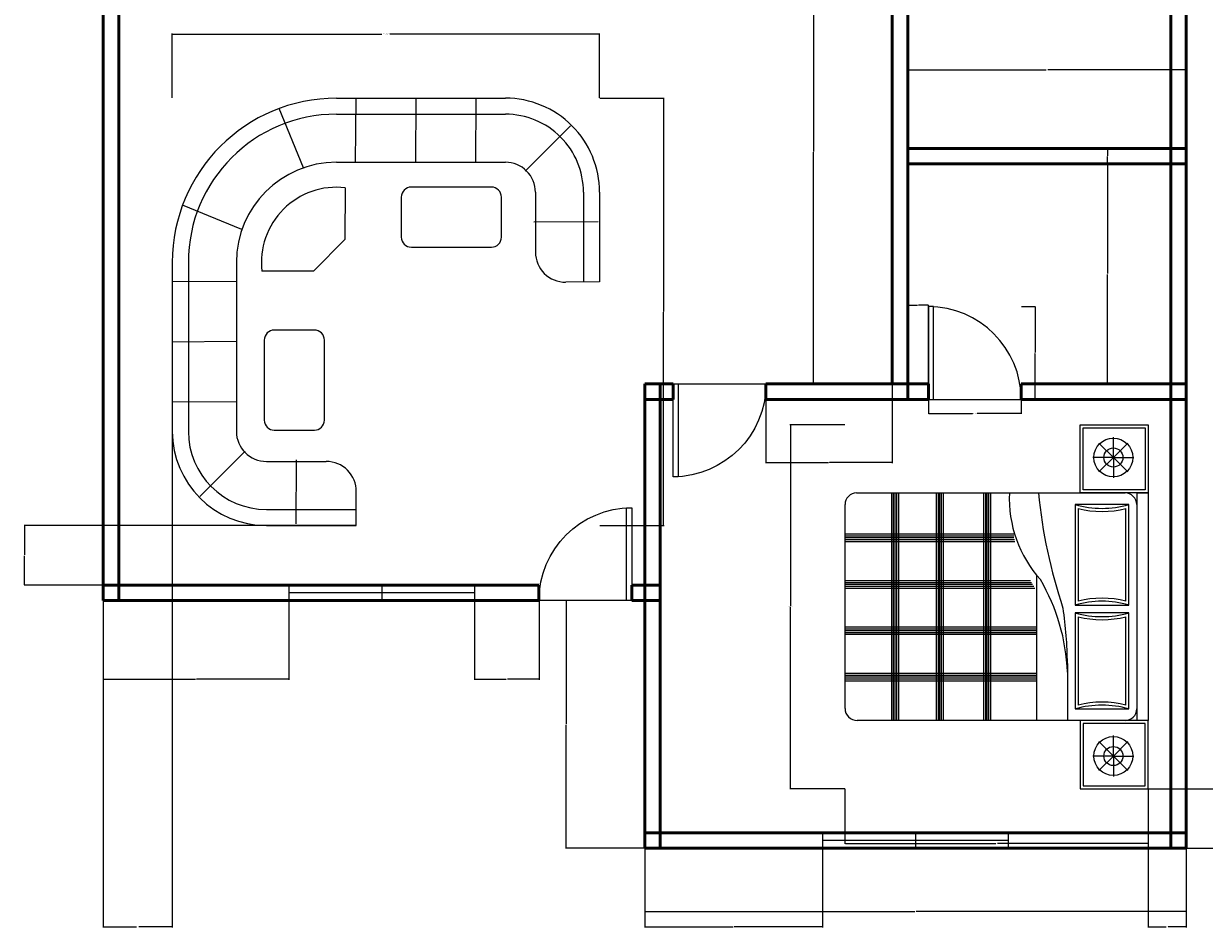
# Model space of a CAD drawing. Units: inches. Extents: x 224 to 929, y 339 to 940.
# Tile 1 of 3: x 224 to 682, y 339 to 689. Entities that reach past the tile are written whole.
import ezdxf

# ---------------------------------------------------------------- set-up
doc = ezdxf.new("R2010")
doc.units = ezdxf.units.IN
for name, color, linetype, lineweight in [('A-ANNO-DIMS', 2, 'Continuous', 18), ('A-DOOR', 3, 'Continuous', 25), ('A-FURN', 8, 'Continuous', 18), ('A-GLAZ', 4, 'Continuous', 18), ('A-WALL', 7, 'Continuous', 50)]:
    doc.layers.add(name, color=color, linetype=linetype, lineweight=lineweight)
doc.styles.get("Standard").update_dxf_attribs({"font": 'arial.ttf'})
doc.dimstyles.get("Standard").update_dxf_attribs({"dimtxt": 0.18, "dimasz": 0.18, "dimexe": 0.18, "dimexo": 0.0625, "dimgap": 0.09, "dimtad": 0, "dimtih": 1, "dimtoh": 1, "dimdec": 4, "dimzin": 0, "dimdsep": 46, "dimtxsty": 'Standard', "dimcen": 0.09, "dimadec": 0, "dimazin": 0, "dimtfac": 1, "dimtdec": 4, "dimtofl": 0, "dimtmove": 0, "dimatfit": 3, "dimfxl": 1, "dimtolj": 1, "dimtzin": 0, "dimarcsym": 0})

# ---------------------------------------------------------------- blocks, each defined once
blk = doc.blocks.new('A$C2EB62172')
at = {"linetype": 'ByBlock'}
for p, q in [((0, 2.0003), (0.45, 2.0003)), ((0, 1.5503), (0, 2.0003)), ((0.45, 1.9241), (0.45, 2.0003)), ((0.45, 2.0003), (0.45, 1.5503)), ((0.45, 2.0003), (1.9506, 2.0003)), ((1.9506, 2.0003), (1.9506, 1.5503)), ((2.4006, 2.0003), (1.9506, 2.0003)), ((2.4006, 1.5503), (2.4006, 2.0003)), ((0.45, 1.9241), (1.9506, 1.9241)), ((0.45, 0.0763), (0.45, 1.8479)), ((1.9506, 1.8479), (1.9506, 0.0801)), ((0.45, 1.5503), (0, 1.5503)), ((1.9506, 1.5503), (2.4006, 1.5503)), ((1.8706, 0.0001), (0.5262, 0.0001))]:
    blk.add_line(p, q, dxfattribs=at)
for p, q in [((0.02, 1.9803), (0.43, 1.9803)), ((0.02, 1.5703), (0.02, 1.9803)), ((0.43, 1.9803), (0.43, 1.5703)), ((1.9706, 1.9803), (1.9706, 1.5703)), ((2.3806, 1.9803), (1.9706, 1.9803)), ((2.3806, 1.5703), (2.3806, 1.9803)), ((0.2161, 1.7703), (0.2161, 1.9047)), ((0.5262, 1.8733), (0.5262, 1.5177)), ((1.1893, 1.8733), (0.5262, 1.8733)), ((1.1893, 1.5177), (1.1893, 1.8733)), ((1.2401, 1.8733), (1.2401, 1.5177)), ((1.8744, 1.8733), (1.2401, 1.8733)), ((1.8744, 1.5177), (1.8744, 1.8733)), ((2.1846, 1.7703), (2.1846, 1.9047)), ((0.2161, 1.7703), (0.1211, 1.8653)), ((0.2161, 1.7703), (0.3111, 1.8653)), ((1.1632, 1.8533), (0.5523, 1.8533)), ((1.8483, 1.8533), (1.2662, 1.8533)), ((2.1846, 1.7703), (2.0896, 1.8653)), ((2.1846, 1.7703), (2.2796, 1.8653)), ((0.2161, 1.7703), (0.0817, 1.7703)), ((0.2161, 1.7703), (0.1211, 1.6753)), ((0.2161, 1.7703), (0.3505, 1.7703)), ((0.2161, 1.7703), (0.3111, 1.6753)), ((0.2161, 1.7703), (0.2161, 1.6359)), ((2.1846, 1.7703), (2.0502, 1.7703)), ((2.1846, 1.7703), (2.0896, 1.6753)), ((2.1846, 1.7703), (2.1846, 1.6359)), ((2.1846, 1.7703), (2.319, 1.7703)), ((2.1846, 1.7703), (2.2796, 1.6753)), ((0.43, 1.5703), (0.02, 1.5703)), ((1.9706, 1.5703), (2.3806, 1.5703)), ((0.5262, 1.5177), (1.1893, 1.5177)), ((0.5523, 1.5377), (1.1632, 1.5377)), ((1.2401, 1.5177), (1.8744, 1.5177)), ((1.2662, 1.5377), (1.8483, 1.5377)), ((1.5747, 1.4669), (1.9506, 1.4669)), ((0.996, 1.2637), (1.9506, 1.2637)), ((1.079, 1.2529), (1.079, 0.0001)), ((1.3351, 1.2637), (1.3351, 0.0001)), ((1.3471, 1.2637), (1.3471, 0.0001)), ((1.3591, 1.2637), (1.3591, 0.0001)), ((1.3722, 1.2637), (1.3722, 0.0001)), ((1.3842, 1.2637), (1.3842, 0.0001)), ((1.6409, 1.2637), (1.6409, 0.0001)), ((1.6529, 1.2637), (1.6529, 0.0001)), ((1.6649, 1.2637), (1.6649, 0.0001)), ((1.678, 1.2637), (1.678, 0.0001)), ((1.69, 1.2637), (1.69, 0.0001)), ((1.0299, 1.2232), (1.0299, 0.0001)), ((1.0419, 1.2301), (1.0419, 0.0001)), ((1.0539, 1.2373), (1.0539, 0.0001)), ((1.067, 1.2453), (1.067, 0.0001)), ((0.722, 1.1147), (0.722, 0.0001)), ((0.734, 1.1147), (0.734, 0.0001)), ((0.746, 1.1147), (0.746, 0.0001)), ((0.7591, 1.1172), (0.7591, 0.0001)), ((0.7711, 1.1203), (0.7711, 0.0001)), ((0.45, 0.9593), (1.9506, 0.9593)), ((0.45, 0.9473), (1.9506, 0.9473)), ((0.45, 0.9353), (1.9506, 0.9353)), ((0.45, 0.9259), (1.9506, 0.9259)), ((0.45, 0.9139), (1.9506, 0.9139)), ((0.45, 0.6471), (1.9506, 0.6471)), ((0.45, 0.6351), (1.9506, 0.6351)), ((0.45, 0.6231), (1.9506, 0.6231)), ((0.45, 0.6137), (1.9506, 0.6137)), ((0.45, 0.6017), (1.9506, 0.6017)), ((0.45, 0.3522), (1.9506, 0.3522)), ((0.45, 0.3402), (1.9506, 0.3402)), ((0.45, 0.3282), (1.9506, 0.3282)), ((0.45, 0.3188), (1.9506, 0.3188)), ((0.45, 0.3068), (1.9506, 0.3068))]:
    blk.add_line(p, q)
for centre, radius in [((0.2161, 1.7703), 0.1285), ((2.1846, 1.7703), 0.1285), ((0.2161, 1.7703), 0.0628), ((2.1846, 1.7703), 0.0628)]:
    blk.add_circle(centre, radius)
for centre, radius, start, end in [((0.5262, 1.8479), 0.0762, 90, 180), ((1.8744, 1.8479), 0.0762, 0, 90), ((1.8706, 0.0801), 0.08, 270, 0), ((0.5262, 0.0763), 0.0762, 180, 270)]:
    blk.add_arc(centre, radius, start, end, dxfattribs=at)
for centre, radius, start, end in [((-0.0834, 1.6955), 0.635, 343.73979, 16.26021), ((1.7989, 1.6955), 0.635, 163.73979, 196.26021), ((0.6305, 1.6955), 0.635, 343.73979, 16.26021), ((2.484, 1.6955), 0.635, 163.73979, 196.26021), ((-0.0834, 1.6955), 0.655, 346.05939, 13.94061), ((1.7989, 1.6955), 0.655, 166.05939, 193.94061), ((0.6305, 1.6955), 0.655, 346.05939, 13.94061), ((2.484, 1.6955), 0.655, 166.05939, 193.94061), ((0.1114, 4.7131), 3.454, 275.6242, 288.5258), ((1.6775, 0.1733), 1.2944, 92.03201, 120.45698), ((1.5739, -0.8648), 2.3317, 89.98016, 99.00664), ((0.4851, 1.8866), 0.8029, 267.49694, 311.91323)]:
    blk.add_arc(centre, radius, start, end)
blk = doc.blocks.new('A$C0BCD5431')
for p, q in [((2628, 4268), (940, 4268)), ((1236, 4268), (1240, 3628)), ((1836, 4268), (1840, 3628)), ((2436, 4268), (2440, 3628)), ((2957, 3573), (3201, 4165)), ((2628, 4108), (940, 4108)), ((742, 3540), (290, 3993)), ((2628, 3628), (940, 3628)), ((0, 3328), (0, 2432)), ((160, 3328), (160, 2431)), ((640, 3328), (640, 2730)), ((1852, 3349), (1052, 3349)), ((2542, 3373), (2545, 2855)), ((952, 3249), (952, 2849)), ((1952, 2849), (1952, 3249)), ((3573, 2957), (4165, 3201)), ((15, 3032), (655, 3028)), ((2545, 2855), (2855, 2545)), ((1052, 2749), (1852, 2749)), ((3628, 2628), (3628, 940)), ((4108, 2628), (4108, 940)), ((4268, 2628), (4268, 940)), ((3373, 2542), (2855, 2545)), ((0, 2432), (338, 2430)), ((4268, 2436), (3628, 2440)), ((3280, 1980), (2880, 1980)), ((2780, 1880), (2780, 1080)), ((3380, 1080), (3380, 1880)), ((4268, 1836), (3628, 1840)), ((4268, 1236), (3628, 1240)), ((2880, 980), (3280, 980)), ((3540, 742), (3993, 290)), ((3328, 640), (2730, 640)), ((3032, 15), (3028, 655)), ((2432, 0), (2430, 338)), ((3328, 160), (2431, 160)), ((3328, 0), (2432, 0))]:
    blk.add_line(p, q)
for centre, radius, start, end in [((940, 3328), 940, 90, 180), ((2628, 2628), 1640, 0, 90), ((940, 3328), 780, 90, 180), ((2628, 2628), 1480, 0, 90), ((940, 3328), 300, 90, 180), ((2628, 2628), 1000, 0, 90), ((1052, 3249), 100, 90, 180), ((1852, 3249), 100, 0, 90), ((2628, 2628), 750, 353.3601, 96.6399), ((1052, 2849), 100, 180, 270), ((1852, 2849), 100, 270, 0), ((340, 2730), 300, 269.6481, 0), ((2880, 1880), 100, 90, 180), ((3280, 1880), 100, 0, 90), ((2880, 1080), 100, 180, 270), ((3280, 1080), 100, 270, 0), ((3328, 940), 300, 270, 0), ((3328, 940), 780, 270, 0), ((3328, 940), 940, 270, 0), ((2730, 340), 300, 90, 180.3519)]:
    blk.add_arc(centre, radius, start, end)
blk = doc.blocks.new('DOOR-SINGLE-36IN')
blk.add_line((0, 0), (36, 0))
blk.add_lwpolyline([(2, 0), (2, 36), (0, 36), (0, 0)], close=True)
blk.add_arc((0, 0), 36, 0, 90)
blk = doc.blocks.new('WIN-72IN')
for p, q in [((0, 0), (0, 6)), ((36, 0), (36, 6)), ((72, 0), (72, 6)), ((0, 3), (72, 3))]:
    blk.add_line(p, q)
blk = doc.blocks.new('*D5')
at = {"layer": 'A-ANNO-DIMS', "color": 0, "lineweight": -2, "transparency": 16777216}
for p, q in [((574.67, 543.56), (574.67, 538.05)), ((610.67, 543.56), (610.67, 538.05)), ((574.85, 538.23), (591.73, 538.23)), ((610.49, 538.23), (593.6, 538.23))]:
    blk.add_line(p, q, dxfattribs=at)
at = {"layer": 'A-ANNO-DIMS', "color": 0, "transparency": 16777216}
for points in [[(574.85, 538.26), (574.85, 538.2), (574.67, 538.23)], [(610.49, 538.26), (610.49, 538.2), (610.67, 538.23)]]:
    blk.add_solid(points, dxfattribs=at)
at = {"layer": 'Defpoints', "color": 0, "transparency": 16777216}
for p in [(574.67, 543.63), (610.67, 543.63), (610.67, 538.23)]:
    blk.add_point(p, dxfattribs=at)
at = {"layer": 'A-ANNO-DIMS', "color": 0, "transparency": 16777216, "insert": (592.67, 538.23), "char_height": 0.18, "attachment_point": 5}
blk.add_mtext('\\A1;DOOR 36 TYP.', dxfattribs=at)
blk = doc.blocks.new('*D6')
at = {"layer": 'A-ANNO-DIMS', "color": 0, "lineweight": -2, "transparency": 16777216}
for p, q in [((610.73, 579.63), (616.25, 579.63)), ((616.07, 579.45), (616.07, 561.81)), ((616.07, 543.81), (616.07, 561.44)), ((610.73, 543.63), (616.25, 543.63))]:
    blk.add_line(p, q, dxfattribs=at)
at = {"layer": 'A-ANNO-DIMS', "color": 0, "transparency": 16777216}
for points in [[(616.04, 579.45), (616.1, 579.45), (616.07, 579.63)], [(616.04, 543.81), (616.1, 543.81), (616.07, 543.63)]]:
    blk.add_solid(points, dxfattribs=at)
at = {"layer": 'Defpoints', "color": 0, "transparency": 16777216}
for p in [(610.67, 579.63), (616.07, 579.63), (610.67, 543.63)]:
    blk.add_point(p, dxfattribs=at)
at = {"layer": 'A-ANNO-DIMS', "color": 0, "transparency": 16777216, "insert": (616.07, 561.63), "char_height": 0.18, "attachment_point": 5}
blk.add_mtext('\\A1;36 TYP.', dxfattribs=at)
blk = doc.blocks.new('*D11')
at = {"layer": 'A-ANNO-DIMS', "color": 0, "lineweight": -2, "transparency": 16777216}
for p, q in [((542.28, 533.81), (520.99, 533.81)), ((521.17, 533.63), (521.17, 463.43)), ((521.17, 392.86), (521.17, 463.06)), ((542.28, 392.68), (520.99, 392.68))]:
    blk.add_line(p, q, dxfattribs=at)
at = {"layer": 'A-ANNO-DIMS', "color": 0, "transparency": 16777216}
for points in [[(521.14, 533.63), (521.2, 533.63), (521.17, 533.81)], [(521.14, 392.86), (521.2, 392.86), (521.17, 392.68)]]:
    blk.add_solid(points, dxfattribs=at)
at = {"layer": 'Defpoints', "color": 0, "transparency": 16777216}
for p in [(542.34, 533.81), (521.17, 392.68), (542.34, 392.68)]:
    blk.add_point(p, dxfattribs=at)
at = {"layer": 'A-ANNO-DIMS', "color": 0, "transparency": 16777216, "insert": (521.17, 463.25), "char_height": 0.18, "attachment_point": 5}
blk.add_mtext('\\A1;BED GROUP 141', dxfattribs=at)
blk = doc.blocks.new('*D12')
at = {"layer": 'A-ANNO-DIMS', "color": 0, "lineweight": -2, "transparency": 16777216}
for p, q in [((542.34, 392.62), (542.34, 371.33)), ((659.94, 392.62), (659.94, 371.33)), ((542.52, 371.51), (600.86, 371.51)), ((659.76, 371.51), (601.42, 371.51))]:
    blk.add_line(p, q, dxfattribs=at)
at = {"layer": 'A-ANNO-DIMS', "color": 0, "transparency": 16777216}
for points in [[(542.52, 371.54), (542.52, 371.48), (542.34, 371.51)], [(659.76, 371.54), (659.76, 371.48), (659.94, 371.51)]]:
    blk.add_solid(points, dxfattribs=at)
at = {"layer": 'Defpoints', "color": 0, "transparency": 16777216}
for p in [(542.34, 392.68), (659.94, 392.68), (659.94, 371.51)]:
    blk.add_point(p, dxfattribs=at)
at = {"layer": 'A-ANNO-DIMS', "color": 0, "transparency": 16777216, "insert": (601.14, 371.51), "char_height": 0.18, "attachment_point": 5}
blk.add_mtext('\\A1;118', dxfattribs=at)
blk = doc.blocks.new('*D13')
at = {"layer": 'A-ANNO-DIMS', "color": 0, "lineweight": -2, "transparency": 16777216}
for p, q in [((281.45, 660.5), (281.45, 685.47)), ((281.63, 685.29), (362.76, 685.29)), ((446.95, 685.29), (365.82, 685.29)), ((447.13, 660.5), (447.13, 685.47))]:
    blk.add_line(p, q, dxfattribs=at)
at = {"layer": 'A-ANNO-DIMS', "color": 0, "transparency": 16777216}
for points in [[(281.63, 685.32), (281.63, 685.26), (281.45, 685.29)], [(446.95, 685.32), (446.95, 685.26), (447.13, 685.29)]]:
    blk.add_solid(points, dxfattribs=at)
at = {"layer": 'Defpoints', "color": 0, "transparency": 16777216}
for p in [(281.45, 685.29), (281.45, 660.43), (447.13, 660.43)]:
    blk.add_point(p, dxfattribs=at)
at = {"layer": 'A-ANNO-DIMS', "color": 0, "transparency": 16777216, "insert": (364.29, 685.29), "char_height": 0.18, "attachment_point": 5}
blk.add_mtext('\\A1;SECTIONAL GROUP 166', dxfattribs=at)
blk = doc.blocks.new('*D14')
at = {"layer": 'A-ANNO-DIMS', "color": 0, "lineweight": -2, "transparency": 16777216}
for p, q in [((447.2, 660.43), (472.16, 660.43)), ((471.98, 660.25), (471.98, 577.77)), ((471.98, 494.93), (471.98, 577.41)), ((447.2, 494.75), (472.16, 494.75))]:
    blk.add_line(p, q, dxfattribs=at)
at = {"layer": 'A-ANNO-DIMS', "color": 0, "transparency": 16777216}
for points in [[(471.95, 660.25), (472.01, 660.25), (471.98, 660.43)], [(471.95, 494.93), (472.01, 494.93), (471.98, 494.75)]]:
    blk.add_solid(points, dxfattribs=at)
at = {"layer": 'Defpoints', "color": 0, "transparency": 16777216}
for p in [(447.13, 660.43), (471.98, 660.43), (447.13, 494.75)]:
    blk.add_point(p, dxfattribs=at)
at = {"layer": 'A-ANNO-DIMS', "color": 0, "transparency": 16777216, "insert": (471.98, 577.59), "char_height": 0.18, "attachment_point": 5}
blk.add_mtext('\\A1;166', dxfattribs=at)
blk = doc.blocks.new('*D16')
at = {"layer": 'A-ANNO-DIMS', "color": 0, "lineweight": -2, "transparency": 16777216}
for p, q in [((668.73, 909.63), (699.35, 909.63)), ((699.17, 909.45), (699.17, 639.81)), ((699.17, 369.81), (699.17, 639.44)), ((668.73, 369.63), (699.35, 369.63))]:
    blk.add_line(p, q, dxfattribs=at)
at = {"layer": 'A-ANNO-DIMS', "color": 0, "transparency": 16777216}
for points in [[(699.14, 909.45), (699.2, 909.45), (699.17, 909.63)], [(699.14, 369.81), (699.2, 369.81), (699.17, 369.63)]]:
    blk.add_solid(points, dxfattribs=at)
at = {"layer": 'Defpoints', "color": 0, "transparency": 16777216}
for p in [(668.67, 909.63), (668.67, 369.63), (699.17, 369.63)]:
    blk.add_point(p, dxfattribs=at)
at = {"layer": 'A-ANNO-DIMS', "color": 0, "transparency": 16777216, "insert": (699.17, 639.63), "char_height": 0.18, "attachment_point": 5}
blk.add_mtext('\\A1;540', dxfattribs=at)
blk = doc.blocks.new('*D20')
at = {"layer": 'A-ANNO-DIMS', "color": 0, "lineweight": -2, "transparency": 16777216}
for p, q in [((464.67, 375.56), (464.67, 344.95)), ((674.67, 375.56), (674.67, 344.95)), ((464.85, 345.13), (569.38, 345.13)), ((674.49, 345.13), (569.96, 345.13))]:
    blk.add_line(p, q, dxfattribs=at)
at = {"layer": 'A-ANNO-DIMS', "color": 0, "transparency": 16777216}
for points in [[(464.85, 345.16), (464.85, 345.1), (464.67, 345.13)], [(674.49, 345.16), (674.49, 345.1), (674.67, 345.13)]]:
    blk.add_solid(points, dxfattribs=at)
at = {"layer": 'Defpoints', "color": 0, "transparency": 16777216}
for p in [(464.67, 375.63), (674.67, 375.63), (464.67, 345.13)]:
    blk.add_point(p, dxfattribs=at)
at = {"layer": 'A-ANNO-DIMS', "color": 0, "transparency": 16777216, "insert": (569.67, 345.13), "char_height": 0.18, "attachment_point": 5}
blk.add_mtext('\\A1;210', dxfattribs=at)
blk = doc.blocks.new('*D21')
at = {"layer": 'A-ANNO-DIMS', "color": 0, "lineweight": -2, "transparency": 16777216}
for p, q in [((464.6, 465.63), (433.99, 465.63)), ((434.17, 465.45), (434.17, 417.81)), ((434.17, 369.81), (434.17, 417.44)), ((464.6, 369.63), (433.99, 369.63))]:
    blk.add_line(p, q, dxfattribs=at)
at = {"layer": 'A-ANNO-DIMS', "color": 0, "transparency": 16777216}
for points in [[(434.14, 465.45), (434.2, 465.45), (434.17, 465.63)], [(434.14, 369.81), (434.2, 369.81), (434.17, 369.63)]]:
    blk.add_solid(points, dxfattribs=at)
at = {"layer": 'Defpoints', "color": 0, "transparency": 16777216}
for p in [(434.17, 465.63), (464.67, 465.63), (464.67, 369.63)]:
    blk.add_point(p, dxfattribs=at)
at = {"layer": 'A-ANNO-DIMS', "color": 0, "transparency": 16777216, "insert": (434.17, 417.63), "char_height": 0.18, "attachment_point": 5}
blk.add_mtext('\\A1;96', dxfattribs=at)
blk = doc.blocks.new('*D22')
at = {"layer": 'A-ANNO-DIMS', "color": 0, "lineweight": -2, "transparency": 16777216}
for p, q in [((254.67, 465.56), (254.67, 434.95)), ((326.67, 465.56), (326.67, 434.95)), ((254.85, 435.13), (290.45, 435.13)), ((326.49, 435.13), (290.88, 435.13))]:
    blk.add_line(p, q, dxfattribs=at)
at = {"layer": 'A-ANNO-DIMS', "color": 0, "transparency": 16777216}
for points in [[(254.85, 435.16), (254.85, 435.1), (254.67, 435.13)], [(326.49, 435.16), (326.49, 435.1), (326.67, 435.13)]]:
    blk.add_solid(points, dxfattribs=at)
at = {"layer": 'Defpoints', "color": 0, "transparency": 16777216}
for p in [(254.67, 465.63), (326.67, 465.63), (254.67, 435.13)]:
    blk.add_point(p, dxfattribs=at)
at = {"layer": 'A-ANNO-DIMS', "color": 0, "transparency": 16777216, "insert": (290.67, 435.13), "char_height": 0.18, "attachment_point": 5}
blk.add_mtext('\\A1;72', dxfattribs=at)
blk = doc.blocks.new('*D23')
at = {"layer": 'A-ANNO-DIMS', "color": 0, "lineweight": -2, "transparency": 16777216}
for p, q in [((398.67, 465.56), (398.67, 434.95)), ((423.67, 465.56), (423.67, 434.95)), ((398.85, 435.13), (410.95, 435.13)), ((423.49, 435.13), (411.39, 435.13))]:
    blk.add_line(p, q, dxfattribs=at)
at = {"layer": 'A-ANNO-DIMS', "color": 0, "transparency": 16777216}
for points in [[(398.85, 435.16), (398.85, 435.1), (398.67, 435.13)], [(423.49, 435.16), (423.49, 435.1), (423.67, 435.13)]]:
    blk.add_solid(points, dxfattribs=at)
at = {"layer": 'Defpoints', "color": 0, "transparency": 16777216}
for p in [(398.67, 465.63), (423.67, 465.63), (398.67, 435.13)]:
    blk.add_point(p, dxfattribs=at)
at = {"layer": 'A-ANNO-DIMS', "color": 0, "transparency": 16777216, "insert": (411.17, 435.13), "char_height": 0.18, "attachment_point": 5}
blk.add_mtext('\\A1;25', dxfattribs=at)
blk = doc.blocks.new('*D24')
at = {"layer": 'A-ANNO-DIMS', "color": 0, "lineweight": -2, "transparency": 16777216}
for p, q in [((464.67, 369.56), (464.67, 338.95)), ((533.67, 369.56), (533.67, 338.95)), ((464.85, 339.13), (498.95, 339.13)), ((533.49, 339.13), (499.39, 339.13))]:
    blk.add_line(p, q, dxfattribs=at)
at = {"layer": 'A-ANNO-DIMS', "color": 0, "transparency": 16777216}
for points in [[(464.85, 339.16), (464.85, 339.1), (464.67, 339.13)], [(533.49, 339.16), (533.49, 339.1), (533.67, 339.13)]]:
    blk.add_solid(points, dxfattribs=at)
at = {"layer": 'Defpoints', "color": 0, "transparency": 16777216}
for p in [(464.67, 369.63), (533.67, 369.63), (464.67, 339.13)]:
    blk.add_point(p, dxfattribs=at)
at = {"layer": 'A-ANNO-DIMS', "color": 0, "transparency": 16777216, "insert": (499.17, 339.13), "char_height": 0.18, "attachment_point": 5}
blk.add_mtext('\\A1;69', dxfattribs=at)
blk = doc.blocks.new('*D25')
at = {"layer": 'A-ANNO-DIMS', "color": 0, "lineweight": -2, "transparency": 16777216}
for p, q in [((560.6, 729.63), (529.99, 729.63)), ((530.17, 729.45), (530.17, 639.81)), ((530.17, 549.81), (530.17, 639.44)), ((560.6, 549.63), (529.99, 549.63))]:
    blk.add_line(p, q, dxfattribs=at)
at = {"layer": 'A-ANNO-DIMS', "color": 0, "transparency": 16777216}
for points in [[(530.14, 729.45), (530.2, 729.45), (530.17, 729.63)], [(530.14, 549.81), (530.2, 549.81), (530.17, 549.63)]]:
    blk.add_solid(points, dxfattribs=at)
at = {"layer": 'Defpoints', "color": 0, "transparency": 16777216}
for p in [(530.17, 729.63), (560.67, 729.63), (560.67, 549.63)]:
    blk.add_point(p, dxfattribs=at)
at = {"layer": 'A-ANNO-DIMS', "color": 0, "transparency": 16777216, "insert": (530.17, 639.63), "char_height": 0.18, "attachment_point": 5}
blk.add_mtext('\\A1;180', dxfattribs=at)
blk = doc.blocks.new('*D26')
at = {"layer": 'A-ANNO-DIMS', "color": 0, "lineweight": -2, "transparency": 16777216}
for p, q in [((674.6, 634.95), (643.99, 634.95)), ((644.17, 634.77), (644.17, 592.47)), ((644.17, 549.81), (644.17, 592.11)), ((674.6, 549.63), (643.99, 549.63))]:
    blk.add_line(p, q, dxfattribs=at)
at = {"layer": 'A-ANNO-DIMS', "color": 0, "transparency": 16777216}
for points in [[(644.14, 634.77), (644.2, 634.77), (644.17, 634.95)], [(644.14, 549.81), (644.2, 549.81), (644.17, 549.63)]]:
    blk.add_solid(points, dxfattribs=at)
at = {"layer": 'Defpoints', "color": 0, "transparency": 16777216}
for p in [(644.17, 634.95), (674.67, 634.95), (674.67, 549.63)]:
    blk.add_point(p, dxfattribs=at)
at = {"layer": 'A-ANNO-DIMS', "color": 0, "transparency": 16777216, "insert": (644.17, 592.29), "char_height": 0.18, "attachment_point": 5}
blk.add_mtext('\\A1;85.33', dxfattribs=at)
blk = doc.blocks.new('*D27')
at = {"layer": 'A-ANNO-DIMS', "color": 0, "lineweight": -2, "transparency": 16777216}
for p, q in [((674.6, 640.95), (643.99, 640.95)), ((644.17, 640.77), (644.17, 638.13)), ((644.17, 635.13), (644.17, 637.77)), ((674.6, 634.95), (643.99, 634.95))]:
    blk.add_line(p, q, dxfattribs=at)
at = {"layer": 'A-ANNO-DIMS', "color": 0, "transparency": 16777216}
for points in [[(644.14, 640.77), (644.2, 640.77), (644.17, 640.95)], [(644.14, 635.13), (644.2, 635.13), (644.17, 634.95)]]:
    blk.add_solid(points, dxfattribs=at)
at = {"layer": 'Defpoints', "color": 0, "transparency": 16777216}
for p in [(644.17, 640.95), (674.67, 640.95), (674.67, 634.95)]:
    blk.add_point(p, dxfattribs=at)
at = {"layer": 'A-ANNO-DIMS', "color": 0, "transparency": 16777216, "insert": (644.17, 637.95), "char_height": 0.18, "attachment_point": 5}
blk.add_mtext('\\A1;6', dxfattribs=at)
blk = doc.blocks.new('*D30')
at = {"layer": 'A-ANNO-DIMS', "color": 0, "lineweight": -2, "transparency": 16777216}
for p, q in [((566.67, 641.01), (566.67, 671.63)), ((566.85, 671.45), (620.39, 671.45)), ((674.49, 671.45), (620.95, 671.45)), ((674.67, 641.01), (674.67, 671.63))]:
    blk.add_line(p, q, dxfattribs=at)
at = {"layer": 'A-ANNO-DIMS', "color": 0, "transparency": 16777216}
for points in [[(566.85, 671.48), (566.85, 671.42), (566.67, 671.45)], [(674.49, 671.48), (674.49, 671.42), (674.67, 671.45)]]:
    blk.add_solid(points, dxfattribs=at)
at = {"layer": 'Defpoints', "color": 0, "transparency": 16777216}
for p in [(674.67, 671.45), (566.67, 640.95), (674.67, 640.95)]:
    blk.add_point(p, dxfattribs=at)
at = {"layer": 'A-ANNO-DIMS', "color": 0, "transparency": 16777216, "insert": (620.67, 671.45), "char_height": 0.18, "attachment_point": 5}
blk.add_mtext('\\A1;108', dxfattribs=at)
blk = doc.blocks.new('*D34')
at = {"layer": 'A-ANNO-DIMS', "color": 0, "lineweight": -2, "transparency": 16777216}
for p, q in [((511.67, 549.56), (511.67, 518.95)), ((560.67, 549.56), (560.67, 518.95)), ((511.85, 519.13), (535.94, 519.13)), ((560.49, 519.13), (536.39, 519.13))]:
    blk.add_line(p, q, dxfattribs=at)
at = {"layer": 'A-ANNO-DIMS', "color": 0, "transparency": 16777216}
for points in [[(511.85, 519.16), (511.85, 519.1), (511.67, 519.13)], [(560.49, 519.16), (560.49, 519.1), (560.67, 519.13)]]:
    blk.add_solid(points, dxfattribs=at)
at = {"layer": 'Defpoints', "color": 0, "transparency": 16777216}
for p in [(511.67, 549.63), (560.67, 549.63), (511.67, 519.13)]:
    blk.add_point(p, dxfattribs=at)
at = {"layer": 'A-ANNO-DIMS', "color": 0, "transparency": 16777216, "insert": (536.17, 519.13), "char_height": 0.18, "attachment_point": 5}
blk.add_mtext('\\A1;49', dxfattribs=at)
blk = doc.blocks.new('*D35')
at = {"layer": 'A-ANNO-DIMS', "color": 0, "lineweight": -2, "transparency": 16777216}
for p, q in [((566.67, 549.69), (566.67, 580.31)), ((566.85, 580.13), (570.52, 580.13)), ((574.49, 580.13), (570.82, 580.13)), ((574.67, 549.69), (574.67, 580.31))]:
    blk.add_line(p, q, dxfattribs=at)
at = {"layer": 'A-ANNO-DIMS', "color": 0, "transparency": 16777216}
for points in [[(566.85, 580.16), (566.85, 580.1), (566.67, 580.13)], [(574.49, 580.16), (574.49, 580.1), (574.67, 580.13)]]:
    blk.add_solid(points, dxfattribs=at)
at = {"layer": 'Defpoints', "color": 0, "transparency": 16777216}
for p in [(574.67, 580.13), (566.67, 549.63), (574.67, 549.63)]:
    blk.add_point(p, dxfattribs=at)
at = {"layer": 'A-ANNO-DIMS', "color": 0, "transparency": 16777216, "insert": (570.67, 580.13), "char_height": 0.18, "attachment_point": 5}
blk.add_mtext('\\A1;8', dxfattribs=at)
blk = doc.blocks.new('*D38')
at = {"layer": 'A-ANNO-DIMS', "color": 0, "lineweight": -2, "transparency": 16777216}
for p, q in [((659.94, 392.62), (659.94, 338.95)), ((674.67, 369.56), (674.67, 338.95)), ((660.12, 339.13), (666.92, 339.13)), ((674.49, 339.13), (667.69, 339.13))]:
    blk.add_line(p, q, dxfattribs=at)
at = {"layer": 'A-ANNO-DIMS', "color": 0, "transparency": 16777216}
for points in [[(660.12, 339.16), (660.12, 339.1), (659.94, 339.13)], [(674.49, 339.16), (674.49, 339.1), (674.67, 339.13)]]:
    blk.add_solid(points, dxfattribs=at)
at = {"layer": 'Defpoints', "color": 0, "transparency": 16777216}
for p in [(659.94, 392.68), (674.67, 369.63), (659.94, 339.13)]:
    blk.add_point(p, dxfattribs=at)
at = {"layer": 'A-ANNO-DIMS', "color": 0, "transparency": 16777216, "insert": (667.3, 339.13), "char_height": 0.18, "attachment_point": 5}
blk.add_mtext('\\A1;14.73', dxfattribs=at)
blk = doc.blocks.new('*D39')
at = {"layer": 'A-ANNO-DIMS', "color": 0, "lineweight": -2, "transparency": 16777216}
for p, q in [((660, 392.68), (705.35, 392.68)), ((705.17, 392.5), (705.17, 381.33)), ((705.17, 369.81), (705.17, 380.97)), ((668.73, 369.63), (705.35, 369.63))]:
    blk.add_line(p, q, dxfattribs=at)
at = {"layer": 'A-ANNO-DIMS', "color": 0, "transparency": 16777216}
for points in [[(705.14, 392.5), (705.2, 392.5), (705.17, 392.68)], [(705.14, 369.81), (705.2, 369.81), (705.17, 369.63)]]:
    blk.add_solid(points, dxfattribs=at)
at = {"layer": 'Defpoints', "color": 0, "transparency": 16777216}
for p in [(659.94, 392.68), (705.17, 392.68), (668.67, 369.63)]:
    blk.add_point(p, dxfattribs=at)
at = {"layer": 'A-ANNO-DIMS', "color": 0, "transparency": 16777216, "insert": (705.17, 381.15), "char_height": 0.18, "attachment_point": 5}
blk.add_mtext('\\A1;23.054', dxfattribs=at)
blk = doc.blocks.new('*D40')
at = {"layer": 'A-ANNO-DIMS', "color": 0, "lineweight": -2, "transparency": 16777216}
for p, q in [((281.45, 531.18), (281.45, 338.95)), ((254.67, 465.56), (254.67, 338.95)), ((254.85, 339.13), (267.59, 339.13)), ((281.27, 339.13), (268.52, 339.13))]:
    blk.add_line(p, q, dxfattribs=at)
at = {"layer": 'A-ANNO-DIMS', "color": 0, "transparency": 16777216}
for points in [[(254.85, 339.16), (254.85, 339.1), (254.67, 339.13)], [(281.27, 339.16), (281.27, 339.1), (281.45, 339.13)]]:
    blk.add_solid(points, dxfattribs=at)
at = {"layer": 'Defpoints', "color": 0, "transparency": 16777216}
for p in [(281.45, 531.24), (254.67, 465.63), (254.67, 339.13)]:
    blk.add_point(p, dxfattribs=at)
at = {"layer": 'A-ANNO-DIMS', "color": 0, "transparency": 16777216, "insert": (268.06, 339.13), "char_height": 0.18, "attachment_point": 5}
blk.add_mtext('\\A1;26.785', dxfattribs=at)
blk = doc.blocks.new('*D41')
at = {"layer": 'A-ANNO-DIMS', "color": 0, "lineweight": -2, "transparency": 16777216}
for p, q in [((352.66, 494.75), (223.99, 494.75)), ((224.17, 494.57), (224.17, 483.37)), ((224.17, 471.81), (224.17, 483.01)), ((326.6, 471.63), (223.99, 471.63))]:
    blk.add_line(p, q, dxfattribs=at)
at = {"layer": 'A-ANNO-DIMS', "color": 0, "transparency": 16777216}
for points in [[(224.14, 494.57), (224.2, 494.57), (224.17, 494.75)], [(224.14, 471.81), (224.2, 471.81), (224.17, 471.63)]]:
    blk.add_solid(points, dxfattribs=at)
at = {"layer": 'Defpoints', "color": 0, "transparency": 16777216}
for p in [(224.17, 494.75), (352.72, 494.75), (326.67, 471.63)]:
    blk.add_point(p, dxfattribs=at)
at = {"layer": 'A-ANNO-DIMS', "color": 0, "transparency": 16777216, "insert": (224.17, 483.19), "char_height": 0.18, "attachment_point": 5}
blk.add_mtext('\\A1;23.126', dxfattribs=at)

msp = doc.modelspace()

# ---------------------------------------------------------------- linework, layer by layer
at = {"layer": 'A-WALL'}
for p, q in [((254.6661, 909.6252), (254.6661, 465.6252)), ((260.6661, 909.6252), (260.6661, 465.6252)), ((668.6661, 369.6252), (668.6661, 909.6252)), ((674.6661, 369.6252), (674.6661, 909.6252)), ((560.6661, 729.6252), (560.6661, 549.6252)), ((566.6661, 729.6252), (566.6661, 549.6252)), ((674.6661, 729.6252), (674.6661, 549.6252)), ((566.6661, 640.9519), (674.6661, 640.9519)), ((566.6661, 634.9519), (674.6661, 634.9519)), ((464.6661, 549.6252), (475.6661, 549.6252)), ((464.6661, 369.6252), (464.6661, 549.6252)), ((470.6661, 369.6252), (470.6661, 549.6252)), ((470.6661, 543.6252), (470.6661, 549.6252)), ((475.6661, 543.6252), (475.6661, 549.6252)), ((511.6661, 543.6252), (511.6661, 549.6252)), ((511.6661, 549.6252), (574.6661, 549.6252)), ((560.6661, 549.6252), (566.6661, 549.6252)), ((566.6661, 549.6252), (566.6661, 543.6252)), ((574.6661, 549.6252), (574.6661, 543.6252)), ((610.6661, 549.6252), (610.6661, 543.6252)), ((610.6661, 549.6252), (674.6661, 549.6252)), ((464.6661, 543.6252), (475.6661, 543.6252)), ((511.6661, 543.6252), (574.6661, 543.6252)), ((610.6661, 543.6252), (674.6661, 543.6252)), ((423.6661, 471.6252), (254.6661, 471.6252)), ((423.6661, 465.6252), (423.6661, 471.6252)), ((470.6661, 471.6252), (459.6661, 471.6252)), ((459.6661, 465.6252), (459.6661, 471.6252)), ((464.6661, 465.6252), (464.6661, 471.6252)), ((423.6661, 465.6252), (254.6661, 465.6252)), ((470.6661, 465.6252), (459.6661, 465.6252)), ((464.6661, 375.6252), (674.6661, 375.6252)), ((464.6661, 369.6252), (674.6661, 369.6252))]:
    msp.add_line(p, q, dxfattribs=at)

# ---------------------------------------------------------------- block references
at = {"layer": 'A-DOOR'}
msp.add_blockref('DOOR-SINGLE-36IN', (574.666, 543.625), dxfattribs=at)
at = {"layer": 'A-DOOR', "extrusion": (0, 0, -1), "zscale": -1, "rotation": 180}
msp.add_blockref('DOOR-SINGLE-36IN', (-475.666, 549.6253), dxfattribs=at)
at = {"layer": 'A-DOOR', "extrusion": (0, 0, -1), "zscale": -1}
msp.add_blockref('DOOR-SINGLE-36IN', (-459.6663, 465.625), dxfattribs=at)
at = {"layer": 'A-FURN'}
for name, p, xscale, yscale, zscale, rotation in [('A$C0BCD5431', (447.1327, 494.7515), 0.0388168482802603, 0.0388168482802603, 0.0388168482802603, 90.00000000000007), ('A$C2EB62172', (542.3367, 533.8151), 58.79096355689981, 58.79096355689981, 58.79096355689981, 270)]:
    msp.add_blockref(name, p, dxfattribs=dict(at, xscale=xscale, yscale=yscale, zscale=zscale, rotation=rotation))
at = {"layer": 'A-GLAZ', "rotation": 180}
for p in [(398.6663, 471.6253), (605.6663, 375.6253)]:
    msp.add_blockref('WIN-72IN', p, dxfattribs=at)

# ---------------------------------------------------------------- dimensions: what is measured, and where the dimension line sits
at = {"layer": 'A-ANNO-DIMS'}
for base, p1, p2, angle, override, picture, middle in [((699.1661, 369.6252), (668.6661, 909.6252), (668.6661, 369.6252), 270, {"dimdec": 0, "dimlfac": 1, "dimrnd": 0, "dimzin": 0, "dimdsep": 46, "dimlunit": 2}, '*D16', (699.1661, 639.6252)), ((530.1661, 729.6252), (560.6661, 549.6252), (560.6661, 729.6252), 90, {"dimdec": 0, "dimlfac": 1, "dimrnd": 0, "dimzin": 0, "dimdsep": 46, "dimlunit": 2}, '*D25', (530.1661, 639.6252)), ((471.9849, 660.4331), (447.1327, 494.7515), (447.1327, 660.4331), 90, {"dimdec": 0, "dimlfac": 1, "dimrnd": 0, "dimzin": 0, "dimdsep": 46, "dimlunit": 2}, '*D14', (471.9849, 577.5923)), ((644.1661, 640.9519), (674.6661, 634.9519), (674.6661, 640.9519), 90, {"dimdec": 0, "dimlfac": 1, "dimrnd": 0, "dimzin": 0, "dimdsep": 46, "dimlunit": 2}, '*D27', (644.1661, 637.9519)), ((644.1661, 634.9519), (674.6661, 549.6252), (674.6661, 634.9519), 90, {"dimdec": 2, "dimlfac": 1, "dimrnd": 0, "dimzin": 0, "dimdsep": 46, "dimlunit": 2}, '*D26', (644.1661, 592.2885)), ((511.6661, 519.1252), (560.6661, 549.6252), (511.6661, 549.6252), 180, {"dimdec": 0, "dimlfac": 1, "dimrnd": 0, "dimzin": 0, "dimdsep": 46, "dimlunit": 2}, '*D34', (536.1661, 519.1252)), ((224.1661, 494.7515), (326.6661, 471.6252), (352.7181, 494.7515), 90, {"dimdec": 3, "dimlfac": 1, "dimrnd": 0, "dimzin": 0, "dimdsep": 46, "dimlunit": 2}, '*D41', (224.1661, 483.1884)), ((254.6661, 435.1252), (326.6661, 465.6252), (254.6661, 465.6252), 180, {"dimdec": 0, "dimlfac": 1, "dimrnd": 0, "dimzin": 0, "dimdsep": 46, "dimlunit": 2}, '*D22', (290.6661, 435.1252)), ((398.6661, 435.1252), (423.6661, 465.6252), (398.6661, 465.6252), 180, {"dimdec": 0, "dimlfac": 1, "dimrnd": 0, "dimzin": 0, "dimdsep": 46, "dimlunit": 2}, '*D23', (411.1661, 435.1252)), ((434.1661, 465.6252), (464.6661, 369.6252), (464.6661, 465.6252), 90, {"dimdec": 0, "dimlfac": 1, "dimrnd": 0, "dimzin": 0, "dimdsep": 46, "dimlunit": 2}, '*D21', (434.1661, 417.6252)), ((705.1661, 392.6791), (668.6661, 369.6252), (659.9364, 392.6791), 90, {"dimdec": 3, "dimlfac": 1, "dimrnd": 0, "dimzin": 0, "dimdsep": 46, "dimlunit": 2}, '*D39', (705.1661, 381.1521)), ((464.6661, 345.1252), (674.6661, 375.6252), (464.6661, 375.6252), 180, {"dimdec": 0, "dimlfac": 1, "dimrnd": 0, "dimzin": 0, "dimdsep": 46, "dimlunit": 2}, '*D20', (569.6661, 345.1252)), ((464.6661, 339.1252), (533.6661, 369.6252), (464.6661, 369.6252), 180, {"dimdec": 0, "dimlfac": 1, "dimrnd": 0, "dimzin": 0, "dimdsep": 46, "dimlunit": 2}, '*D24', (499.1661, 339.1252))]:
    dim = msp.add_linear_dim(base=base, p1=p1, p2=p2, angle=angle, dimstyle='Standard', override=override, dxfattribs=at)
    dim.commit()
    dim.dimension.update_dxf_attribs({"geometry": picture, "text_midpoint": middle})
for base, p1, p2, angle, text, picture, middle in [((281.4511, 685.2854), (447.1327, 660.4331), (281.4511, 660.4331), 180, 'SECTIONAL GROUP <>', '*D13', (364.2919, 685.2854)), ((616.0661, 579.6252), (610.6661, 543.6252), (610.6661, 579.6252), 90, '<> TYP.', '*D6', (616.0661, 561.6252)), ((521.1727, 392.6791), (542.3427, 533.8127), (542.3427, 392.6791), 270, 'BED GROUP <>', '*D11', (521.1727, 463.2459))]:
    dim = msp.add_linear_dim(base=base, p1=p1, p2=p2, angle=angle, text=text, dimstyle='Standard', override={"dimdec": 0, "dimlfac": 1, "dimrnd": 0, "dimzin": 0, "dimdsep": 46, "dimlunit": 2}, dxfattribs=at)
    dim.commit()
    dim.dimension.update_dxf_attribs({"geometry": picture, "text_midpoint": middle})
for base, p1, p2, override, picture, middle in [((674.6661, 671.4519), (566.6661, 640.9519), (674.6661, 640.9519), {"dimdec": 0, "dimlfac": 1, "dimrnd": 0, "dimzin": 0, "dimdsep": 46, "dimlunit": 2}, '*D30', (620.6661, 671.4519)), ((574.6661, 580.1252), (566.6661, 549.6252), (574.6661, 549.6252), {"dimdec": 0, "dimlfac": 1, "dimrnd": 0, "dimzin": 0, "dimdsep": 46, "dimlunit": 2}, '*D35', (570.6661, 580.1252)), ((254.6661, 339.1252), (281.4511, 531.2394), (254.6661, 465.6252), {"dimdec": 3, "dimlfac": 1, "dimrnd": 0, "dimzin": 0, "dimdsep": 46, "dimlunit": 2}, '*D40', (268.0586, 339.1252)), ((659.9364, 371.509), (542.3427, 392.6791), (659.9364, 392.6791), {"dimdec": 0, "dimlfac": 1, "dimrnd": 0, "dimzin": 0, "dimdsep": 46, "dimlunit": 2}, '*D12', (601.1396, 371.509)), ((659.9364, 339.1252), (674.6661, 369.6252), (659.9364, 392.6791), {"dimdec": 2, "dimlfac": 1, "dimrnd": 0, "dimzin": 0, "dimdsep": 46, "dimlunit": 2}, '*D38', (667.3013, 339.1252))]:
    dim = msp.add_linear_dim(base=base, p1=p1, p2=p2, dimstyle='Standard', override=override, dxfattribs=at)
    dim.commit()
    dim.dimension.update_dxf_attribs({"geometry": picture, "text_midpoint": middle})
dim = msp.add_linear_dim(base=(610.6661, 538.2252), p1=(574.6661, 543.6252), p2=(610.6661, 543.6252), text='DOOR <> TYP.', dimstyle='Standard', override={"dimdec": 0, "dimlfac": 1, "dimrnd": 0, "dimzin": 0, "dimdsep": 46, "dimlunit": 2}, dxfattribs=at)
dim.commit()
dim.dimension.update_dxf_attribs({"geometry": '*D5', "text_midpoint": (592.6661, 538.2252)})

doc.saveas('drawing.dxf')
